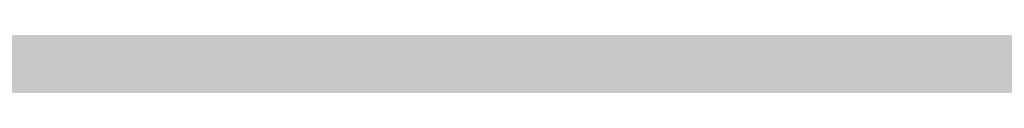
# Model space of a CAD drawing. Units: inches. Extents: x 2091 to 2899, y 967 to 2217.
# Tile 216 of 256: x 2203.2571 to 2203.4104, y 1152.2538 to 1152.2605. Entities that reach past the tile are written whole.
import ezdxf

# ---------------------------------------------------------------- set-up
doc = ezdxf.new("R2010")
doc.units = ezdxf.units.IN
doc.layers.add('A-WALL-PATT', color=141, linetype='Continuous', lineweight=13, true_color=0xadddf7)

msp = doc.modelspace()

# ---------------------------------------------------------------- hatches: boundary and pattern name
at = {"layer": 'A-WALL-PATT'}
h = msp.add_hatch(color=256, dxfattribs=at)
h.dxf.hatch_style = 1
h.paths.add_polyline_path([(2803.1436, 2050.91906), (2203.1436, 2050.91906), (2203.1436, 1090.91906), (2803.1436, 1090.91906)])
h.paths.add_polyline_path([(2635.79885, 1147.54046), (2674.52405, 1147.54046, 0.376086), (2678.52967, 1152.8802), (2678.52967, 1159.55647, 0.333335), (2674.52432, 1163.56185), (2674.52432, 1163.56185), (2674.52432, 1192.93439), (2635.80597, 1192.93439), (2597.08762, 1192.93439), (2597.08762, 1163.56185, 0.333335), (2593.08228, 1159.55647), (2593.08228, 1152.8802, 0.376086), (2597.08789, 1147.54046)], flags=0)
h.paths.add_polyline_path([(2436.01043, 1278.24078, 0.000483), (2435.95264, 1278.21503, -0.001328), (2435.93563, 1278.11169, -0.001711), (2436.11644, 1278.04076, 0.002185)], flags=0)
h.paths.add_polyline_path([(2794.1436, 1143.41906), (2794.1436, 1347.41906), (2543.37017, 1347.41906), (2543.37017, 1351.91906), (2794.1436, 1351.91906), (2794.1436, 1392.71355), (2793.9474, 1392.71355), (2793.9474, 1473.5369), (2794.1436, 1473.5369), (2794.1436, 1531.91906), (2650.1436, 1531.91906), (2650.1436, 1536.41906), (2794.1436, 1536.41906), (2794.1436, 1692.41906), (2609.37561, 1692.41906), (2609.37561, 1644.41906), (2604.87561, 1644.41906), (2604.87561, 1744.91906), (2609.37561, 1744.91906), (2609.37561, 1696.91906), (2794.1436, 1696.91906), (2794.1436, 1780.91906), (2609.6436, 1780.91906), (2493.87561, 1780.91906), (2493.87561, 1785.41906), (2609.6436, 1785.41906), (2794.1436, 1785.41906), (2794.1436, 1847.93882), (2793.95122, 1847.93882), (2793.95122, 1928.76217), (2794.1436, 1928.76217), (2794.1436, 1941.41906), (2614.1436, 1941.41906), (2614.1436, 1821.41906), (2609.6436, 1821.41906), (2609.6436, 1941.41906), (2392.1436, 1941.41906), (2392.1436, 1819.91906), (2387.6436, 1819.91906), (2387.6436, 1941.41906), (2212.1436, 1941.41906), (2212.1436, 1783.91906), (2392.1436, 1783.91906), (2392.1436, 1780.91906), (2212.1436, 1780.91906), (2212.1436, 1629.41906), (2387.6436, 1629.41906), (2387.6436, 1744.91906), (2392.1436, 1744.91906), (2392.1436, 1627.91906), (2317.1436, 1627.91906), (2317.1436, 1551.41906), (2317.1436, 1536.41906), (2459.38359, 1536.41906), (2459.38359, 1602.39648), (2463.88359, 1602.39648), (2463.88359, 1531.91906), (2456.6436, 1531.91906), (2456.6436, 1529.91906), (2452.1436, 1529.91906), (2452.1436, 1531.91906), (2312.6436, 1531.91906), (2312.6436, 1551.41906), (2306.1436, 1551.41906), (2306.1436, 1555.91906), (2308.1436, 1555.91906), (2308.1436, 1551.41906), (2312.6436, 1551.41906), (2312.6436, 1627.91906), (2212.1436, 1627.91906), (2212.1436, 1555.91906), (2270.1436, 1555.91906), (2270.1436, 1551.41906), (2212.1436, 1551.41906), (2212.1436, 1351.91906), (2272.1436, 1351.91906), (2272.1436, 1347.41906), (2212.1436, 1347.41906), (2212.1436, 1275.41906), (2308.1436, 1275.41906), (2308.1436, 1351.91906), (2452.1436, 1351.91906), (2452.1436, 1493.91906), (2456.6436, 1493.91906), (2456.6436, 1347.41906), (2312.6436, 1347.41906), (2312.6436, 1270.91906), (2212.1436, 1270.91906), (2212.1436, 1099.91906), (2281.23752, 1099.91906), (2282.87104, 1110.9138), (2282.00834, 1116.9966), (2278.55774, 1121.4204), (2268.20564, 1128.0562), (2272.08764, 1128.0562), (2273.81294, 1131.927), (2279.42034, 1134.6919), (2285.02784, 1135.2449), (2287.61584, 1137.4568), (2288.04714, 1138.0098), (2289.34114, 1140.7747), (2291.06654, 1139.6687), (2292.36054, 1135.2449), (2295.37984, 1136.9038), (2296.24254, 1135.7979), (2297.10524, 1133.033), (2300.12464, 1138.0098), (2303.14394, 1138.0098), (2304.43794, 1135.7979), (2303.14394, 1133.586), (2306.59464, 1134.6919), (2307.88874, 1133.033), (2310.90804, 1135.2449), (2313.92744, 1134.1389), (2315.62686, 1132.4271), (2308.32004, 1117.5496), (2290.20384, 1109.8079), (2288.90984, 1103.1721), (2289.27231, 1099.91906), (2434.91823, 1099.91906), (2431.59323, 1124.78806), (2429.93023, 1169.55306), (2430.92718, 1240.51969), (2435.65893, 1238.18613), (2437.13523, 1196.55406), (2438.79823, 1143.97306), (2442.67823, 1111.99806), (2446.55823, 1099.91906), (2794.1436, 1099.91906), (2794.1436, 1138.91906), (2548.03245, 1138.91906), (2548.03245, 1143.41906), (2548.03245, 1148.81906), (2546.66846, 1148.03156), (2528.68569, 1179.17862, 0.256256), (2512.03245, 1148.81906), (2512.03245, 1143.41906), (2512.03245, 1138.91906), (2507.53245, 1138.91906), (2507.53245, 1143.41906), (2507.53245, 1148.81906, 0.256256), (2490.8792, 1179.17862), (2472.89644, 1148.03156), (2471.53245, 1148.81906), (2471.53245, 1143.41906), (2467.03245, 1143.41906), (2467.03245, 1269.94579, 0.039061), (2460.90999, 1273.58006), (2467.03245, 1273.58006), (2467.03245, 1286.32536, 0.014511), (2465.21619, 1286.76191), (2467.03245, 1287.05258), (2467.03245, 1323.41906), (2471.53245, 1323.41906), (2471.53245, 1148.81906), (2489.53245, 1179.99597), (2490.89644, 1179.20847), (2490.8792, 1179.17862, -0.256256), (2507.53245, 1148.81906), (2507.53245, 1143.41906), (2512.03245, 1143.41906), (2512.03245, 1148.81906, -0.256256), (2528.68569, 1179.17862), (2528.66846, 1179.20847), (2530.03245, 1179.99597), (2548.03245, 1148.81906), (2548.03245, 1143.41906)], flags=16)
h.paths.add_polyline_path([(2607.76855, 1200.94508), (2607.76855, 1265.03063), (2597.08762, 1281.05201), (2619.78459, 1281.05201), (2627.79528, 1337.12686), (2635.79885, 1337.12686), (2643.81666, 1337.12686), (2651.82736, 1281.05201), (2674.52432, 1281.05201), (2663.8434, 1265.03063), (2663.8434, 1200.94508), (2635.80597, 1200.94508)], flags=0)
edge = h.paths.add_edge_path(flags=0)
edge.add_ellipse((13303.89622, 1272.99872), major_axis=(-10595.31304, 0), ratio=0.84230387009, start_angle=0.628237219, end_angle=0.6465541, ccw=False)
edge.add_ellipse((2711.70045, 1156.85268), major_axis=(2.21977, 0), ratio=0.8423039, start_angle=111.53524, end_angle=180.62824, ccw=False)
edge.add_ellipse((13303.15629, 1272.99872), major_axis=(-10593.02631, 0), ratio=0.84230386954, start_angle=0.528271472, end_angle=0.646554097, ccw=False)
edge.add_line((2710.7646, 1175.3333), (2710.12999, 1175.3333))
edge.add_ellipse((2710.12999, 1176.57978), major_axis=(1.47985, 0), ratio=0.8423039, start_angle=180, end_angle=270, ccw=False)
edge.add_line((2708.65014, 1176.57978), (2708.65014, 1200.78291))
edge.add_ellipse((2710.12999, 1200.78291), major_axis=(1.47985, 0), ratio=0.8423039, start_angle=90, end_angle=180, ccw=False)
edge.add_line((2710.12999, 1202.02939), (2710.46508, 1202.02939))
edge.add_ellipse((13303.15629, 1272.99872), major_axis=(-10593.02631, 0), ratio=0.84230386954, start_angle=-0.090229089, end_angle=0.383866779, ccw=False)
edge.add_ellipse((2710.12999, 1290.92703), major_axis=(-1.47985, 0), ratio=0.8423039, start_angle=0, end_angle=90, ccw=False)
edge.add_line((2708.65014, 1290.92703), (2708.65014, 1315.13017))
edge.add_ellipse((2710.12999, 1315.13017), major_axis=(-1.47985, 0), ratio=0.8423039, start_angle=-90, end_angle=0, ccw=False)
edge.add_line((2710.12999, 1316.37665), (2710.70631, 1316.37665))
edge.add_ellipse((3238.40172, 1296.28957), major_axis=(528.234, 0), ratio=0.84230387, start_angle=176.3495724, end_angle=177.8200497, ccw=False)
edge.add_ellipse((2775.06304, 1071.4507), major_axis=(313.30776, 0), ratio=0.84230387, start_angle=102.1259656, end_angle=103.780529, ccw=False)
edge.add_ellipse((2775.06304, 1078.3057), major_axis=(-305.30289, 0), ratio=0.84230387, start_angle=-79.790461, end_angle=-77.5553727, ccw=False)
edge.add_ellipse((2695.14177, 1541.97538), major_axis=(-250.96022, 0), ratio=0.84230387, start_angle=99.256566, end_angle=102.5549326)
edge.add_line((2741.41033, 1334.21426), (2747.13255, 1337.37848))
edge.add_ellipse((2747.53862, 1336.85748), major_axis=(-0.73992, 0), ratio=0.842304, start_angle=270, end_angle=307.93313, ccw=False)
edge.add_ellipse((2747.53862, 1336.85748), major_axis=(-0.73992, 0), ratio=0.842304, start_angle=232.06687, end_angle=270, ccw=False)
edge.add_line((2747.94469, 1337.37848), (2753.66691, 1334.21426))
edge.add_ellipse((2799.93547, 1541.97538), major_axis=(250.96022, 0), ratio=0.84230387, start_angle=257.4450674, end_angle=260.743434)
edge.add_ellipse((2720.01419, 1078.3057), major_axis=(305.30289, 0), ratio=0.84230387, start_angle=77.5553727, end_angle=79.790461, ccw=False)
edge.add_ellipse((2720.01419, 1071.4507), major_axis=(-313.30776, 0), ratio=0.84230387, start_angle=256.219471, end_angle=257.8740344, ccw=False)
edge.add_ellipse((2256.67551, 1296.28957), major_axis=(-528.234, 0), ratio=0.84230387, start_angle=182.1799503, end_angle=183.6504276, ccw=False)
edge.add_line((2784.37092, 1316.37665), (2784.94725, 1316.37665))
edge.add_ellipse((2784.94725, 1315.13017), major_axis=(1.47985, 0), ratio=0.8423039, start_angle=0, end_angle=90, ccw=False)
edge.add_line((2786.42709, 1315.13017), (2786.42709, 1290.92703))
edge.add_ellipse((2784.94725, 1290.92703), major_axis=(1.47985, 0), ratio=0.8423039, start_angle=270, end_angle=360, ccw=False)
edge.add_ellipse((-7808.07906, 1272.99872), major_axis=(10593.02631, 0), ratio=0.84230386954, start_angle=-0.383866779, end_angle=0.090229089, ccw=False)
edge.add_line((2784.61216, 1202.02939), (2784.94725, 1202.02939))
edge.add_ellipse((2784.94725, 1200.78291), major_axis=(1.47985, 0), ratio=0.8423039, start_angle=0, end_angle=90, ccw=False)
edge.add_line((2786.42709, 1200.78291), (2786.42709, 1176.57978))
edge.add_ellipse((2784.94725, 1176.57978), major_axis=(-1.47985, 0), ratio=0.8423039, start_angle=90, end_angle=180, ccw=False)
edge.add_line((2784.94725, 1175.3333), (2784.31264, 1175.3333))
edge.add_ellipse((-7808.07906, 1272.99872), major_axis=(10593.02631, 0), ratio=0.84230386954, start_angle=-0.618643196, end_angle=-0.528271472, ccw=False)
edge.add_ellipse((2783.37678, 1156.85268), major_axis=(-2.21977, 0), ratio=0.8423039, start_angle=179.37176, end_angle=248.46476, ccw=False)
edge.add_ellipse((-7808.81898, 1272.99872), major_axis=(-10595.31304, 0), ratio=0.84230386576, start_angle=179.353445923, end_angle=179.371762803, ccw=False)
edge.add_ellipse((2780.2973, 1153.50079), major_axis=(-5.24643, 0), ratio=0.8423039, start_angle=90, end_angle=179.35345, ccw=False)
edge.add_line((2780.2973, 1149.08171), (2714.77993, 1149.08171))
edge.add_ellipse((2714.77993, 1153.50079), major_axis=(5.24643, 0), ratio=0.8423039, start_angle=180.64655, end_angle=270, ccw=False)
edge = h.paths.add_edge_path(flags=0)
edge.add_line((2718.18737, 1151.00783), (2718.18737, 1170.47236))
edge.add_ellipse((2721.14706, 1170.47236), major_axis=(-2.95969, 0), ratio=0.8423039, start_angle=-90, end_angle=0, ccw=False)
edge.add_line((2721.14706, 1172.96532), (2773.93017, 1172.96532))
edge.add_ellipse((2773.93017, 1170.47236), major_axis=(-2.95969, 0), ratio=0.8423039, start_angle=180, end_angle=270, ccw=False)
edge.add_line((2776.88987, 1170.47236), (2776.88987, 1151.00783))
edge.add_line((2776.88987, 1151.00783), (2718.18737, 1151.00783))
edge = h.paths.add_edge_path(flags=0)
edge.add_line((2718.18737, 1180.23415), (2718.18737, 1199.05783))
edge.add_ellipse((2747.53862, 1320.39864), major_axis=(147.01792, 0), ratio=0.84230387, start_angle=256.4018653, end_angle=283.5981347)
edge.add_line((2776.88987, 1199.05783), (2776.88987, 1180.23415))
edge.add_ellipse((2747.53862, 1301.57496), major_axis=(147.01792, 0), ratio=0.84230387, start_angle=256.4018653, end_angle=283.5981347, ccw=False)
edge = h.paths.add_edge_path(flags=0)
edge.add_ellipse((13303.15629, 1272.99872), major_axis=(-10591.54646, 0), ratio=0.84230386955, start_angle=0.055594314, end_angle=0.377764194, ccw=False)
edge.add_line((2711.61686, 1262.72171), (2715.66741, 1249.4954))
edge.add_ellipse((6413.89196, 1241.69192), major_axis=(-3698.23616, 0), ratio=0.8423038695, start_angle=-0.12089737, end_angle=0.36407635)
edge.add_line((2715.76104, 1218.19245), (2711.93431, 1203.16736))
edge = h.paths.add_edge_path(flags=0)
edge.add_line((2718.18737, 1251.07457), (2716.00249, 1267.45044))
edge.add_ellipse((2742.15117, 1202.18954), major_axis=(81.77258, 0), ratio=0.84230387, start_angle=94.277421, end_angle=111.8349538, ccw=False)
edge.add_line((2737.00975, 1270.93063), (2758.06748, 1270.93063))
edge.add_ellipse((2752.92606, 1202.18954), major_axis=(81.77258, 0), ratio=0.84230387, start_angle=68.1650462, end_angle=85.722579, ccw=False)
edge.add_line((2779.07475, 1267.45044), (2776.88987, 1251.07457))
edge.add_ellipse((2750.33806, 1187.88536), major_axis=(79.57966, 0), ratio=0.84230387, start_angle=67.2080851, end_angle=85.1299304)
edge.add_line((2756.03466, 1254.74366), (2739.04258, 1254.74366))
edge.add_ellipse((2744.73917, 1187.88536), major_axis=(79.57966, 0), ratio=0.84230387, start_angle=94.8700696, end_angle=112.7919149)
edge = h.paths.add_edge_path(flags=0)
edge.add_line((2783.14293, 1203.16736), (2779.31619, 1218.19245))
edge.add_ellipse((-918.81473, 1241.69192), major_axis=(3698.23616, 0), ratio=0.8423038695, start_angle=-0.36407635, end_angle=0.12089737)
edge.add_line((2779.40983, 1249.4954), (2783.46037, 1262.72171))
edge.add_ellipse((-7808.07906, 1272.99872), major_axis=(-10591.54646, 0), ratio=0.84230386954, start_angle=179.622235806, end_angle=179.944405687, ccw=False)
edge = h.paths.add_edge_path(flags=0)
edge.add_ellipse((2734.20089, 1286.69044), major_axis=(-0.35661, 6.34008), ratio=0.6038336, start_angle=89.002014, end_angle=253.657408, ccw=False)
edge.add_line((2730.369, 1286.54181), (2730.369, 1301.35198))
edge.add_line((2730.369, 1301.35198), (2735.91331, 1305.2148))
edge.add_ellipse((2736.38492, 1304.73456), major_axis=(0.73992, 0), ratio=0.842304, start_angle=90, end_angle=134.48021, ccw=False)
edge.add_line((2736.38492, 1305.3578), (2738.03278, 1305.3578))
edge.add_line((2738.03278, 1305.3578), (2738.03278, 1307.70793))
edge.add_ellipse((2794.20164, 1307.70793), major_axis=(56.16886, 0), ratio=0.84230387, start_angle=150.56143, end_angle=180, ccw=False)
edge.add_ellipse((2700.87559, 1307.70793), major_axis=(-56.16886, 0), ratio=0.84230387, start_angle=180, end_angle=209.43857, ccw=False)
edge.add_line((2757.04445, 1307.70793), (2757.04445, 1305.3578))
edge.add_line((2757.04445, 1305.3578), (2758.69232, 1305.3578))
edge.add_ellipse((2758.69232, 1304.73456), major_axis=(-0.73992, 0), ratio=0.842304, start_angle=225.51979, end_angle=270, ccw=False)
edge.add_line((2759.16392, 1305.2148), (2764.70823, 1301.35198))
edge.add_line((2764.70823, 1301.35198), (2764.70823, 1286.54181))
edge.add_ellipse((2760.87634, 1286.69044), major_axis=(0.35661, 6.34008), ratio=0.6038336, start_angle=106.342592, end_angle=270.997986, ccw=False)
edge.add_line((2757.04445, 1285.79709), (2757.04445, 1307.70793))
edge.add_ellipse((2700.87559, 1307.70793), major_axis=(-56.16886, 0), ratio=0.84230387, start_angle=180, end_angle=209.43857)
edge.add_ellipse((2794.20164, 1307.70793), major_axis=(56.16886, 0), ratio=0.84230387, start_angle=150.56143, end_angle=180)
edge.add_line((2738.03278, 1307.70793), (2738.03278, 1285.79709))
h.paths.add_polyline_path([(2417.81227, 1104.4497), (2413.49227, 1102.5297), (2410.61227, 1103.9697), (2409.17227, 1106.3697), (2407.25227, 1107.3297), (2406.29227, 1109.7297), (2405.33227, 1114.0497), (2405.33227, 1117.8897), (2406.29227, 1120.1297), (2407.25227, 1119.8097), (2408.84832, 1118.32766), (2410.17395, 1119.42417), (2410.21127, 1120.4057), (2411.04073, 1121.41905), (2410.69927, 1119.8587), (2410.17395, 1119.42417), (2410.08845, 1117.17611), (2411.13284, 1116.20632), (2413.97227, 1119.3297), (2416.85227, 1120.7697), (2416.86972, 1120.79878), (2417.03507, 1119.40512), (2417.89621, 1118.14338), (2418.29227, 1118.3697), (2419.54445, 1120.03927), (2419.36092, 1118.38749), (2419.03211, 1119.35615), (2418.39894, 1118.51193), (2419.25227, 1114.5297), (2418.79409, 1107.19879)], flags=0)
h.paths.add_polyline_path([(2508.87017, 1347.41906), (2508.37017, 1347.41906), (2508.37017, 1351.91906), (2508.87017, 1351.91906)], flags=0)
h.paths.add_polyline_path([(2473.37017, 1347.41906), (2472.37017, 1347.41906), (2467.87017, 1347.41906), (2467.87017, 1455.41906), (2472.37017, 1455.41906), (2472.37017, 1352.41906), (2473.37017, 1352.41906)], flags=0)
h.paths.add_polyline_path([(2352.10624, 1217.4462), (2349.22624, 1218.8862), (2347.78624, 1221.2862), (2345.86624, 1222.2462), (2344.90624, 1224.6462), (2343.94624, 1228.9662), (2343.94624, 1232.8062), (2344.90624, 1235.0462), (2345.86624, 1234.7262), (2347.46229, 1233.24415), (2348.78792, 1234.34066), (2348.82524, 1235.3222), (2349.6547, 1236.33555), (2349.31324, 1234.7752), (2348.78792, 1234.34066), (2348.70242, 1232.0926), (2349.74681, 1231.12282), (2352.58624, 1234.2462), (2355.46624, 1235.6862), (2355.48369, 1235.71528), (2355.64904, 1234.32161), (2356.51018, 1233.05988), (2356.90624, 1233.2862), (2358.15842, 1234.95576), (2357.97489, 1233.30398), (2357.64608, 1234.27264), (2357.01291, 1233.42842), (2357.86624, 1229.4462), (2357.40806, 1222.11529), (2356.42624, 1219.3662)], flags=0)
h.paths.add_polyline_path([(2348.2968, 1112.22442), (2347.0138, 1112.31042), (2345.5298, 1114.12742), (2345.7318, 1115.85842), (2346.8118, 1116.98242), (2346.8118, 1114.64642), (2345.8668, 1114.21442), (2346.8798, 1114.30042)], flags=0)
h.paths.add_polyline_path([(2347.0138, 1110.92642), (2346.2718, 1110.49342), (2346.6098, 1111.18642)], flags=0)
h.paths.add_polyline_path([(2345.8668, 1118.19442), (2345.5298, 1117.32942), (2343.7078, 1118.02142), (2344.3828, 1118.62642)], flags=0)
h.paths.add_polyline_path([(2346.6768, 1109.28242), (2346.0698, 1108.07142), (2345.8668, 1110.06142)], flags=0)
h.paths.add_polyline_path([(2345.0568, 1119.75142), (2343.6398, 1119.75142), (2343.9778, 1121.13542)], flags=0)
h.paths.add_polyline_path([(2345.2598, 1116.55042), (2345.1248, 1115.85842), (2344.9218, 1115.68542), (2344.7198, 1116.37742)], flags=0)
h.paths.add_polyline_path([(2345.6648, 1112.31042), (2345.4618, 1111.53242), (2344.0448, 1111.96442), (2344.6518, 1112.57042)], flags=0)
h.paths.add_polyline_path([(2345.1918, 1113.34942), (2344.4498, 1113.86842), (2344.7198, 1114.38742)], flags=0)
h.paths.add_polyline_path([(2344.6518, 1116.80942), (2344.1798, 1115.68542), (2344.6518, 1115.33942), (2343.9098, 1114.90642), (2343.0328, 1115.94442), (2343.6398, 1116.46342)], flags=0)
h.paths.add_polyline_path([(2345.8668, 1106.68642), (2344.9898, 1105.56242), (2344.5168, 1106.60042)], flags=0)
h.paths.add_polyline_path([(2344.8548, 1110.06142), (2344.5168, 1109.28242), (2344.1128, 1109.71542)], flags=0)
h.paths.add_polyline_path([(2344.0448, 1113.52242), (2343.4378, 1113.08942), (2342.7628, 1113.95442)], flags=0)
h.paths.add_polyline_path([(2344.3148, 1111.01242), (2342.9648, 1110.32042), (2342.9648, 1111.09942)], flags=0)
h.paths.add_polyline_path([(2345.1248, 1104.69742), (2344.5848, 1103.74542), (2344.4498, 1104.26442)], flags=0)
h.paths.add_polyline_path([(2342.8298, 1121.22242), (2341.7498, 1120.53042), (2340.5358, 1121.04942), (2340.1308, 1121.82842), (2340.6708, 1122.95242), (2341.1428, 1121.82842), (2341.6148, 1122.00142)], flags=0)
h.paths.add_polyline_path([(2342.9648, 1119.75142), (2343.0328, 1118.45342), (2342.0878, 1118.02142), (2342.0198, 1119.49142)], flags=0)
h.paths.add_polyline_path([(2342.6948, 1116.89642), (2341.9528, 1116.63642), (2342.0198, 1117.32942)], flags=0)
h.paths.add_polyline_path([(2343.0328, 1112.22442), (2342.0198, 1111.79142), (2341.5478, 1112.22442), (2342.3578, 1113.34942)], flags=0)
h.paths.add_polyline_path([(2343.7748, 1104.43742), (2342.6278, 1102.88042), (2342.6948, 1104.61042), (2343.4378, 1105.12942)], flags=0)
h.paths.add_polyline_path([(2342.0198, 1115.07942), (2340.8058, 1115.51242), (2340.9408, 1116.37742)], flags=0)
h.paths.add_polyline_path([(2341.4808, 1120.09742), (2341.4808, 1119.40542), (2341.0758, 1119.57842), (2341.1428, 1120.09742)], flags=0)
h.paths.add_polyline_path([(2341.8178, 1114.47342), (2340.9408, 1113.08942), (2340.8058, 1114.56042)], flags=0)
h.paths.add_polyline_path([(2341.1428, 1118.54042), (2340.9408, 1116.98242), (2339.0508, 1117.67542), (2339.0508, 1118.62642)], flags=0)
h.paths.add_polyline_path([(2342.6948, 1101.66842), (2341.9528, 1101.84142), (2342.5598, 1102.36142)], flags=0)
h.paths.add_polyline_path([(2340.3328, 1119.66542), (2338.4438, 1119.57842), (2337.9038, 1120.35742), (2339.6578, 1120.61642)], flags=0)
h.paths.add_polyline_path([(2340.3328, 1115.33942), (2340.0628, 1113.69542), (2339.3878, 1115.33942)], flags=0)
h.paths.add_polyline_path([(2341.8178, 1103.83142), (2341.5478, 1102.88042), (2341.1428, 1103.65842)], flags=0)
h.paths.add_polyline_path([(2339.0508, 1122.86642), (2337.2958, 1121.82842), (2337.0938, 1123.12542), (2337.7688, 1123.81842)], flags=0)
h.paths.add_polyline_path([(2339.1178, 1121.74142), (2338.8478, 1121.22242), (2338.1738, 1121.04942), (2338.3758, 1121.56842)], flags=0)
h.paths.add_polyline_path([(2339.1858, 1119.31942), (2338.6458, 1118.71342), (2338.2408, 1118.10742), (2338.2408, 1118.88642)], flags=0)
h.paths.add_polyline_path([(2341.1428, 1101.92842), (2340.6028, 1101.23642), (2340.0628, 1101.84142), (2340.6028, 1102.36142)], flags=0)
h.paths.add_polyline_path([(2337.6338, 1117.76142), (2336.6208, 1118.28042), (2337.2958, 1118.97242)], flags=0)
h.paths.add_polyline_path([(2336.8238, 1119.57842), (2334.7988, 1118.97242), (2335.2038, 1120.35742), (2336.5538, 1120.87642)], flags=0)
h.paths.add_polyline_path([(2339.1178, 1100.45742), (2337.3638, 1100.54342), (2336.7558, 1101.23642)], flags=0)
h.paths.add_polyline_path([(2336.3508, 1122.43342), (2336.0138, 1121.91442), (2334.9338, 1122.43342), (2334.5288, 1123.47142), (2335.7438, 1122.77942)], flags=0)
h.paths.add_polyline_path([(2334.7318, 1120.87642), (2334.2588, 1120.35742), (2334.0568, 1120.78942), (2334.5968, 1121.30842)], flags=0)
h.paths.add_polyline_path([(2334.4618, 1122.17442), (2332.5718, 1121.30842), (2331.3568, 1122.17442), (2332.0998, 1122.86642)], flags=0)
h.paths.add_polyline_path([(2334.2588, 1118.54042), (2333.3818, 1118.45342), (2333.6518, 1119.31942)], flags=0)
h.paths.add_polyline_path([(2335.5418, 1102.27442), (2334.1918, 1102.62042), (2335.2718, 1103.31242)], flags=0)
h.paths.add_polyline_path([(2332.7068, 1119.66542), (2331.6948, 1120.44342), (2332.5048, 1120.78942)], flags=0)
h.paths.add_polyline_path([(2334.7318, 1101.14942), (2333.5168, 1101.58242), (2333.9888, 1101.75542)], flags=0)
h.paths.add_polyline_path([(2332.6398, 1116.63642), (2331.0868, 1116.29042), (2331.9648, 1118.19442)], flags=0)
h.paths.add_polyline_path([(2330.7498, 1121.56842), (2330.2768, 1120.27042), (2328.5228, 1119.31942), (2328.9948, 1121.04942)], flags=0)
h.paths.add_polyline_path([(2330.7498, 1118.62642), (2330.0078, 1117.50242), (2329.8728, 1118.02142)], flags=0)
h.paths.add_polyline_path([(2332.0998, 1102.36142), (2330.5468, 1102.01442), (2331.6948, 1102.96642)], flags=0)
h.paths.add_polyline_path([(2329.5348, 1113.60842), (2329.0628, 1112.31042), (2328.5898, 1113.34942)], flags=0)
h.paths.add_polyline_path([(2328.3878, 1117.84842), (2327.5098, 1116.55042), (2327.1728, 1117.76142)], flags=0)
h.paths.add_polyline_path([(2329.7378, 1106.51342), (2329.5348, 1105.30242), (2328.2528, 1106.08142)], flags=0)
h.paths.add_polyline_path([(2328.6578, 1114.38742), (2328.0498, 1114.12742), (2328.3198, 1114.90642)], flags=0)
h.paths.add_polyline_path([(2328.3198, 1112.22442), (2327.1058, 1112.13742), (2326.7008, 1112.65642)], flags=0)
h.paths.add_polyline_path([(2326.9028, 1115.25242), (2326.7008, 1114.12742), (2325.2158, 1113.60842), (2326.0928, 1115.33942)], flags=0)
h.paths.add_polyline_path([(2326.6328, 1108.33042), (2326.0928, 1107.37942), (2325.8908, 1108.50342), (2326.4978, 1109.10942)], flags=0)
h.paths.add_polyline_path([(2615.1436, 1531.91906), (2609.6436, 1531.91906), (2609.6436, 1620.41906), (2614.1436, 1620.41906), (2614.1436, 1536.41906), (2615.1436, 1536.41906)], flags=0)
h.paths.add_polyline_path([(2545.1436, 1563.41906), (2464.1436, 1563.41906), (2464.1436, 1632.41906), (2509.1436, 1632.41906), (2509.1436, 1627.91906), (2509.1436, 1603.91906), (2468.6436, 1603.91906), (2468.6436, 1567.91906), (2540.6436, 1567.91906), (2540.6436, 1591.91906), (2545.1436, 1591.91906)], flags=0)
h.paths.add_polyline_path([(2388.96905, 1549.98573), (2357.43418, 1549.98573), (2357.43418, 1623.36078), (2399.36278, 1623.36078), (2435.68947, 1623.36078), (2435.59255, 1602.55927), (2435.59255, 1602.39648), (2388.96905, 1602.39648)], flags=0)
h.paths.add_polyline_path([(2388.88063, 1555.80915), (2374.90443, 1555.80915), (2374.90443, 1600.57156), (2374.90443, 1615.45765), (2406.35088, 1615.45765), (2406.35088, 1618.93943), (2412.17429, 1615.45765), (2406.35088, 1611.97586), (2406.35088, 1615.45765), (2388.88063, 1615.45765)], flags=0)
h.paths.add_polyline_path([(2568.87561, 1644.41906), (2453.37561, 1644.41906), (2453.37561, 1785.41906), (2457.87561, 1785.41906), (2457.87561, 1648.91906), (2568.87561, 1648.91906)], flags=0)
h.paths.add_polyline_path([(2212.1436, 1945.91906), (2212.1436, 2041.91906), (2794.1436, 2041.91906), (2794.1436, 1945.91906)], flags=16)
h.paths.add_polyline_path([(2271.08273, 1964.31724), (2776.85297, 1964.31724), (2776.85297, 2037.16962), (2271.08273, 2037.16962)], flags=8)
h.paths.add_polyline_path([(2380.64929, 1536.82414), (2461.04081, 1536.82414), (2461.04081, 1554.65259), (2380.64929, 1554.65259)], flags=8)
h.paths.add_polyline_path([(2240.75571, 1609.72545), (2309.18583, 1609.72545), (2309.18583, 1617.6982), (2240.75571, 1617.6982)], flags=8)
h.paths.add_polyline_path([(2212.67726, 1313.5041), (2282.59152, 1313.5041), (2282.59152, 1322.74524), (2212.67726, 1322.74524)], flags=8)
h.paths.add_polyline_path([(2457.11198, 1114.77857), (2558.48158, 1114.77857), (2558.48158, 1142.21968), (2457.11198, 1142.21968)], flags=8)
h.paths.add_polyline_path([(2473.44234, 1273.01007), (2604.64123, 1273.01007), (2604.64123, 1318.34693), (2473.44234, 1318.34693)], flags=8)
h.paths.add_polyline_path([(2638.8763, 1626.97743), (2684.25037, 1627.97674), (2684.03848, 1637.59749), (2638.66442, 1636.59819)], flags=8)
h.paths.add_polyline_path([(2537.59055, 1453.79345), (2628.38955, 1453.79345), (2628.38955, 1475.34481), (2537.59055, 1475.34481)], flags=8)
h.paths.add_polyline_path([(2504.13764, 1714.6324), (2554.64719, 1714.6324), (2554.64719, 1730.23771), (2504.13764, 1730.23771)], flags=8)
h.paths.add_polyline_path([(2487.50118, 1575.65187), (2535.09712, 1575.65187), (2535.09712, 1598.37765), (2487.50118, 1598.37765)], flags=8)
h.paths.add_polyline_path([(2709.0994, 1735.71028), (2740.0166, 1735.71028), (2740.0166, 1749.93764), (2709.0994, 1749.93764)], flags=8)
h.paths.add_polyline_path([(2442.43842, 1792.17166), (2564.72884, 1792.17166), (2564.72884, 1842.00016), (2442.43842, 1842.00016)], flags=8)
h.paths.add_polyline_path([(2655.8158, 1809.64408), (2789.52014, 1806.6938), (2790.08498, 1832.29164), (2656.38064, 1835.24192)], flags=8)
h.paths.add_polyline_path([(2234.8427, 1797.72014), (2368.59285, 1794.76885), (2369.16072, 1820.50413), (2235.41056, 1823.45542)], flags=8)
h.paths.add_polyline_path([(2245.13847, 1644.00633), (2398.42773, 1640.6239), (2398.99484, 1666.32482), (2245.70557, 1669.70725)], flags=8)
h.paths.add_polyline_path([(2306.14285, 1431.16852), (2413.76831, 1428.79369), (2414.33315, 1454.39153), (2306.70768, 1456.76636)], flags=8)
h.paths.add_polyline_path([(2306.83458, 1458.23314), (2393.38048, 1456.32345), (2393.93281, 1481.35436), (2307.38691, 1483.26405)], flags=8)

doc.saveas('drawing.dxf')
